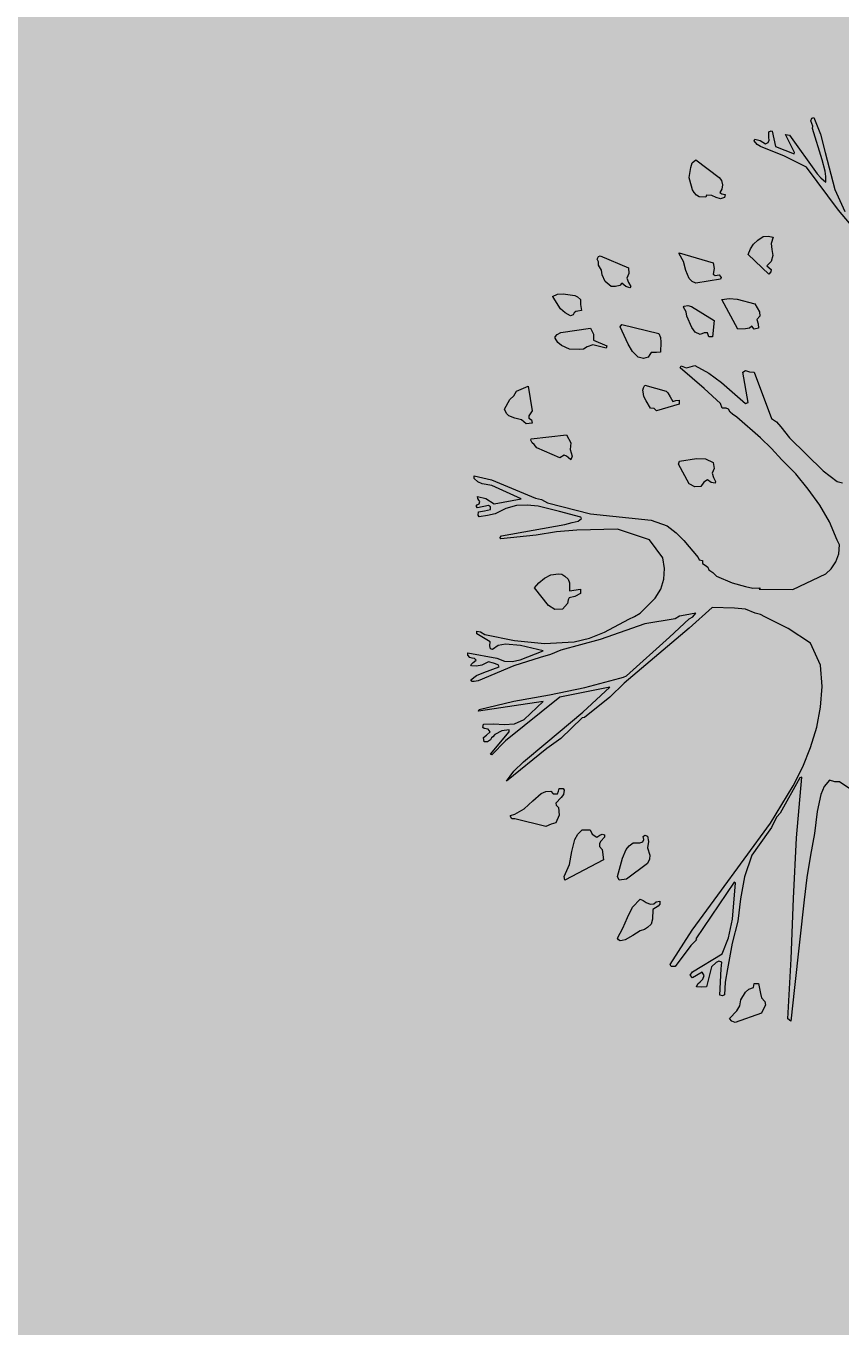
# Model space of a CAD drawing. Units: inches. Extents: x 84 to 1044, y -280 to 906.
# Tile 101 of 105: x 861 to 882, y 478 to 510. Entities that reach past the tile are written whole.
import ezdxf

# ---------------------------------------------------------------- set-up
doc = ezdxf.new("R2010")
doc.units = ezdxf.units.IN
doc.layers.add('A-ANNO-DIMS', color=2, linetype='Continuous', lineweight=18)
doc.layers.add('L-PLNT', color=114, linetype='Continuous', lineweight=15)
doc.layers.add('L-PLNT-PATT', color=9, linetype='Continuous', lineweight=9, true_color=0xafd9aa)
doc.styles.get("Standard").update_dxf_attribs({"font": 'arial.ttf'})
doc.dimstyles.get("Standard").update_dxf_attribs({"dimtxt": 0.18, "dimasz": 0.18, "dimexe": 0.18, "dimexo": 0.0625, "dimgap": 0.09, "dimtad": 0, "dimtih": 1, "dimtoh": 1, "dimdec": 4, "dimzin": 0, "dimdsep": 46, "dimtxsty": 'Standard', "dimcen": 0.09, "dimadec": 0, "dimazin": 0, "dimtfac": 1, "dimtdec": 4, "dimtofl": 0, "dimtmove": 0, "dimatfit": 3, "dimfxl": 1, "dimtolj": 1, "dimtzin": 0, "dimarcsym": 0})

# ---------------------------------------------------------------- blocks, each defined once
blk = doc.blocks.new('A$C37E508DF')
for p, q in [((0.5583, 1.4948), (0.5596, 1.4995)), ((0.5596, 1.4905), (0.5583, 1.4948)), ((0.5596, 1.4995), (0.563, 1.5003)), ((0.5613, 1.4862), (0.5596, 1.4905)), ((0.5608, 1.4823), (0.5613, 1.4862)), ((0.5767, 1.4317), (0.5608, 1.4823)), ((0.563, 1.5003), (0.5737, 1.4733)), ((0.4657, 1.4622), (0.4669, 1.4652)), ((0.4708, 1.4566), (0.4657, 1.4622)), ((0.4669, 1.4652), (0.4755, 1.463)), ((0.4755, 1.463), (0.4845, 1.4575)), ((0.4884, 1.4596), (0.4905, 1.4635)), ((0.4897, 1.4772), (0.4935, 1.4789)), ((0.4897, 1.4678), (0.4897, 1.4772)), ((0.4905, 1.4635), (0.4897, 1.4678)), ((0.4935, 1.4789), (0.4952, 1.478)), ((0.4952, 1.478), (0.5004, 1.4532)), ((0.5313, 1.4437), (0.5167, 1.4729)), ((0.5167, 1.4729), (0.5231, 1.4716)), ((0.5231, 1.4716), (0.5686, 1.409)), ((0.5737, 1.4733), (0.5814, 1.4437)), ((0.4764, 1.4532), (0.4708, 1.4566)), ((0.5154, 1.4373), (0.4764, 1.4532)), ((0.4845, 1.4575), (0.4884, 1.4596)), ((0.5004, 1.4532), (0.5308, 1.4412)), ((0.5308, 1.4412), (0.5313, 1.4437)), ((0.5814, 1.4437), (0.5969, 1.3833)), ((0.3598, 1.403), (0.3628, 1.4189)), ((0.3628, 1.4189), (0.3649, 1.4266)), ((0.3649, 1.4266), (0.3709, 1.4317)), ((0.3709, 1.4317), (0.4086, 1.403)), ((0.551, 1.4197), (0.5154, 1.4373)), ((0.6029, 1.3494), (0.551, 1.4197)), ((0.5814, 1.4133), (0.5767, 1.4317)), ((0.3602, 1.4021), (0.3598, 1.403)), ((0.364, 1.3888), (0.3602, 1.4021)), ((0.4086, 1.403), (0.4125, 1.3979)), ((0.4125, 1.3979), (0.4142, 1.391)), ((0.5686, 1.409), (0.5741, 1.4021)), ((0.5741, 1.4021), (0.5823, 1.3953)), ((0.5827, 1.4043), (0.5814, 1.4133)), ((0.5823, 1.3953), (0.5827, 1.4043)), ((0.3657, 1.3828), (0.364, 1.3888)), ((0.3683, 1.3781), (0.3657, 1.3828)), ((0.3718, 1.3738), (0.3683, 1.3781)), ((0.4134, 1.3837), (0.4099, 1.3781)), ((0.4099, 1.3781), (0.4134, 1.376)), ((0.4142, 1.391), (0.4134, 1.3837)), ((0.4134, 1.376), (0.4189, 1.3751)), ((0.5969, 1.3833), (0.6132, 1.3472)), ((0.3765, 1.3713), (0.3718, 1.3738)), ((0.3872, 1.3708), (0.3765, 1.3713)), ((0.3885, 1.3738), (0.3872, 1.3708)), ((0.3971, 1.3734), (0.3885, 1.3738)), ((0.4039, 1.3704), (0.3971, 1.3734)), ((0.4108, 1.3683), (0.4039, 1.3704)), ((0.4176, 1.37), (0.4108, 1.3683)), ((0.4189, 1.3751), (0.4176, 1.37)), ((0.6595, 1.2829), (0.6029, 1.3494)), ((0.4597, 1.2868), (0.4648, 1.2945)), ((0.4648, 1.2945), (0.4717, 1.3009)), ((0.4717, 1.3009), (0.4807, 1.3065)), ((0.4807, 1.3065), (0.4884, 1.3074)), ((0.4884, 1.3074), (0.4965, 1.3057)), ((0.4965, 1.3057), (0.4935, 1.2954)), ((0.4935, 1.2954), (0.4948, 1.2855)), ((0.2101, 1.2696), (0.2127, 1.2744)), ((0.2127, 1.2744), (0.2152, 1.2752)), ((0.2152, 1.2752), (0.2611, 1.2559)), ((0.3439, 1.2804), (0.3992, 1.2636)), ((0.3439, 1.2787), (0.3439, 1.2804)), ((0.3507, 1.2662), (0.3439, 1.2787)), ((0.4562, 1.2774), (0.4597, 1.2868)), ((0.4897, 1.2452), (0.4562, 1.2774)), ((0.4961, 1.2756), (0.4935, 1.2658)), ((0.4948, 1.2855), (0.4961, 1.2756)), ((0.2127, 1.2654), (0.2101, 1.2696)), ((0.2127, 1.2602), (0.2127, 1.2654)), ((0.2174, 1.2521), (0.2127, 1.2602)), ((0.2182, 1.2443), (0.2174, 1.2521)), ((0.2611, 1.2559), (0.262, 1.2465)), ((0.3546, 1.2516), (0.3507, 1.2662)), ((0.3602, 1.2383), (0.3546, 1.2516)), ((0.3992, 1.2636), (0.4005, 1.2546)), ((0.4005, 1.2546), (0.3992, 1.2452)), ((0.4935, 1.2658), (0.4867, 1.2589)), ((0.4867, 1.2589), (0.4935, 1.2529)), ((0.4931, 1.2491), (0.4897, 1.2452)), ((0.4935, 1.2529), (0.4931, 1.2491)), ((0.2234, 1.2336), (0.2182, 1.2443)), ((0.2328, 1.2251), (0.2234, 1.2336)), ((0.2504, 1.2306), (0.2474, 1.2268)), ((0.2568, 1.2255), (0.2504, 1.2306)), ((0.262, 1.2465), (0.2586, 1.2388)), ((0.2586, 1.2388), (0.2611, 1.2319)), ((0.2611, 1.2319), (0.265, 1.2251)), ((0.3649, 1.2336), (0.3602, 1.2383)), ((0.3709, 1.2306), (0.3649, 1.2336)), ((0.4112, 1.2375), (0.3709, 1.2306)), ((0.3992, 1.2452), (0.4026, 1.2431)), ((0.4026, 1.2431), (0.4086, 1.2443)), ((0.4086, 1.2443), (0.4121, 1.2401)), ((0.4121, 1.2401), (0.4112, 1.2375)), ((0.1376, 1.2092), (0.1458, 1.2126)), ((0.1389, 1.2079), (0.1376, 1.2092)), ((0.1505, 1.189), (0.1389, 1.2079)), ((0.1458, 1.2126), (0.1548, 1.2135)), ((0.1548, 1.2135), (0.1741, 1.2109)), ((0.1741, 1.2109), (0.1784, 1.2083)), ((0.1784, 1.2083), (0.1831, 1.204)), ((0.2401, 1.2251), (0.2328, 1.2251)), ((0.2474, 1.2268), (0.2401, 1.2251)), ((0.2633, 1.2229), (0.2568, 1.2255)), ((0.265, 1.2251), (0.2633, 1.2229)), ((0.1582, 1.1822), (0.1505, 1.189)), ((0.1788, 1.1852), (0.1758, 1.1847)), ((0.1848, 1.1865), (0.1788, 1.1852)), ((0.1831, 1.204), (0.1831, 1.1959)), ((0.1831, 1.1959), (0.1848, 1.1865)), ((0.3507, 1.1916), (0.352, 1.1933)), ((0.355, 1.1839), (0.3507, 1.1916)), ((0.352, 1.1933), (0.3576, 1.1942)), ((0.3576, 1.1942), (0.364, 1.1929)), ((0.364, 1.1929), (0.4005, 1.1702)), ((0.4134, 1.204), (0.4258, 1.2058)), ((0.4391, 1.156), (0.4134, 1.204)), ((0.4258, 1.2058), (0.4382, 1.2045)), ((0.4382, 1.2045), (0.4669, 1.1972)), ((0.4669, 1.1972), (0.4747, 1.1843)), ((0.1668, 1.1775), (0.1582, 1.1822)), ((0.1711, 1.1792), (0.1668, 1.1775)), ((0.1728, 1.1826), (0.1711, 1.1792)), ((0.1758, 1.1847), (0.1728, 1.1826)), ((0.3563, 1.177), (0.355, 1.1839)), ((0.3645, 1.1586), (0.3563, 1.177)), ((0.4005, 1.1702), (0.3979, 1.1436)), ((0.4751, 1.177), (0.47, 1.1714)), ((0.47, 1.1714), (0.4721, 1.1646)), ((0.4721, 1.1646), (0.473, 1.1573)), ((0.4747, 1.1843), (0.4751, 1.177)), ((0.1419, 1.1436), (0.1449, 1.1474)), ((0.1419, 1.141), (0.1419, 1.1436)), ((0.1449, 1.1474), (0.1509, 1.1504)), ((0.1509, 1.1504), (0.1994, 1.1573)), ((0.1994, 1.1573), (0.2041, 1.1479)), ((0.2041, 1.1479), (0.2045, 1.138)), ((0.2478, 1.1594), (0.2504, 1.1637)), ((0.2607, 1.1316), (0.2478, 1.1594)), ((0.2504, 1.1637), (0.3104, 1.1487)), ((0.3104, 1.1487), (0.3134, 1.1423)), ((0.37, 1.1509), (0.3645, 1.1586)), ((0.3778, 1.1474), (0.37, 1.1509)), ((0.3842, 1.15), (0.3778, 1.1474)), ((0.3898, 1.15), (0.3842, 1.15)), ((0.3923, 1.1436), (0.3898, 1.15)), ((0.3979, 1.1436), (0.3923, 1.1436)), ((0.4519, 1.1564), (0.4391, 1.156)), ((0.458, 1.1573), (0.4519, 1.1564)), ((0.4622, 1.1607), (0.458, 1.1573)), ((0.4657, 1.156), (0.4622, 1.1607)), ((0.473, 1.1573), (0.4657, 1.156)), ((0.1462, 1.1342), (0.1419, 1.141)), ((0.1522, 1.1294), (0.1462, 1.1342)), ((0.1655, 1.1234), (0.1522, 1.1294)), ((0.181, 1.1226), (0.1655, 1.1234)), ((0.1878, 1.1234), (0.181, 1.1226)), ((0.1938, 1.1273), (0.1878, 1.1234)), ((0.2032, 1.1303), (0.1938, 1.1273)), ((0.2247, 1.1251), (0.2032, 1.1303)), ((0.2045, 1.138), (0.226, 1.129)), ((0.226, 1.129), (0.2247, 1.1251)), ((0.268, 1.1196), (0.2607, 1.1316)), ((0.3134, 1.1423), (0.3139, 1.1346)), ((0.3139, 1.1346), (0.3134, 1.1183)), ((0.277, 1.1101), (0.268, 1.1196)), ((0.2856, 1.108), (0.277, 1.1101)), ((0.2933, 1.1101), (0.2856, 1.108)), ((0.2959, 1.1144), (0.2933, 1.1101)), ((0.2984, 1.1179), (0.2959, 1.1144)), ((0.3066, 1.1179), (0.2984, 1.1179)), ((0.3134, 1.1183), (0.3066, 1.1179)), ((0.3456, 1.093), (0.3469, 1.0964)), ((0.3842, 1.0591), (0.3456, 1.093)), ((0.3469, 1.0964), (0.355, 1.093)), ((0.355, 1.093), (0.3619, 1.0943)), ((0.3619, 1.0943), (0.3692, 1.0968)), ((0.3692, 1.0968), (0.3923, 1.0844)), ((0.3923, 1.0844), (0.4129, 1.069)), ((0.4472, 1.0857), (0.4515, 1.0887)), ((0.4562, 1.0364), (0.4472, 1.0857)), ((0.4515, 1.0887), (0.4584, 1.0865)), ((0.4584, 1.0865), (0.4657, 1.0861)), ((0.4657, 1.0861), (0.4939, 1.0107)), ((0.0789, 1.0552), (0.0978, 1.063)), ((0.0978, 1.063), (0.1042, 1.0231)), ((0.2847, 1.0565), (0.2856, 1.0604)), ((0.2856, 1.0604), (0.2877, 1.0647)), ((0.2877, 1.0647), (0.3224, 1.0552)), ((0.4112, 1.0351), (0.3842, 1.0591)), ((0.4129, 1.069), (0.4515, 1.0351)), ((0.0596, 1.0257), (0.0682, 1.0415)), ((0.0682, 1.0415), (0.0746, 1.0475)), ((0.0746, 1.0475), (0.0789, 1.0552)), ((0.2851, 1.054), (0.2847, 1.0565)), ((0.2864, 1.0463), (0.2851, 1.054)), ((0.2899, 1.039), (0.2864, 1.0463)), ((0.2972, 1.0274), (0.2899, 1.039)), ((0.3224, 1.0552), (0.3255, 1.0522)), ((0.3255, 1.0522), (0.3293, 1.0458)), ((0.3293, 1.0458), (0.3336, 1.0381)), ((0.3336, 1.0381), (0.3383, 1.0398)), ((0.3383, 1.0398), (0.3439, 1.0402)), ((0.3439, 1.0402), (0.3439, 1.0338)), ((0.0626, 1.0188), (0.0596, 1.0257)), ((0.0665, 1.0149), (0.0626, 1.0188)), ((0.1012, 1.018), (0.099, 1.0149)), ((0.1042, 1.0231), (0.1012, 1.018)), ((0.3032, 1.0265), (0.2972, 1.0274)), ((0.3066, 1.0231), (0.3032, 1.0265)), ((0.3439, 1.0338), (0.3066, 1.0231)), ((0.4138, 1.0274), (0.4112, 1.0351)), ((0.4202, 1.0274), (0.4138, 1.0274)), ((0.4241, 1.0257), (0.4202, 1.0274)), ((0.4267, 1.0209), (0.4241, 1.0257)), ((0.4305, 1.0175), (0.4267, 1.0209)), ((0.4378, 1.0124), (0.4305, 1.0175)), ((0.4515, 1.0351), (0.4562, 1.0364)), ((0.0763, 1.0111), (0.0665, 1.0149)), ((0.087, 1.0085), (0.0763, 1.0111)), ((0.0948, 1.0016), (0.087, 1.0085)), ((0.1042, 1.0029), (0.0948, 1.0016)), ((0.099, 1.0149), (0.099, 1.0111)), ((0.099, 1.0111), (0.1033, 1.0085)), ((0.1033, 1.0085), (0.1042, 1.0029)), ((0.476, 0.9789), (0.4378, 1.0124)), ((0.4939, 1.0107), (0.5021, 1.0051)), ((0.5021, 1.0051), (0.5094, 0.9969)), ((0.5094, 0.9969), (0.5231, 0.9789)), ((0.1025, 0.9751), (0.1029, 0.9772)), ((0.1046, 0.9708), (0.1025, 0.9751)), ((0.1029, 0.9772), (0.1604, 0.9841)), ((0.1604, 0.9841), (0.1672, 0.9708)), ((0.4939, 0.9618), (0.476, 0.9789)), ((0.5231, 0.9789), (0.578, 0.9253)), ((0.1076, 0.9682), (0.1046, 0.9708)), ((0.1119, 0.9626), (0.1076, 0.9682)), ((0.1496, 0.9463), (0.1119, 0.9626)), ((0.1672, 0.9708), (0.1664, 0.9601)), ((0.1664, 0.9601), (0.1698, 0.9493)), ((0.5111, 0.9429), (0.4939, 0.9618)), ((0.1565, 0.9506), (0.1496, 0.9463)), ((0.1604, 0.9493), (0.1565, 0.9506)), ((0.1629, 0.9468), (0.1604, 0.9493)), ((0.1672, 0.9429), (0.1629, 0.9468)), ((0.1698, 0.9493), (0.1672, 0.9429)), ((0.3426, 0.936), (0.3443, 0.9412)), ((0.3602, 0.9039), (0.3426, 0.936)), ((0.3443, 0.9412), (0.3722, 0.9451)), ((0.3722, 0.9451), (0.3868, 0.9446)), ((0.3868, 0.9446), (0.3992, 0.9386)), ((0.3992, 0.9386), (0.4009, 0.9292)), ((0.5334, 0.9202), (0.5111, 0.9429)), ((0.0103, 0.9129), (0.0103, 0.9172)), ((0.0103, 0.9172), (0.0382, 0.9107)), ((0.0159, 0.9073), (0.0103, 0.9129)), ((0.0382, 0.9107), (0.1098, 0.8807)), ((0.3898, 0.9107), (0.3838, 0.9069)), ((0.3958, 0.906), (0.3898, 0.9107)), ((0.4009, 0.9292), (0.3975, 0.9215)), ((0.3975, 0.9215), (0.3996, 0.9142)), ((0.3996, 0.9142), (0.4031, 0.9077)), ((0.554, 0.8953), (0.5334, 0.9202)), ((0.578, 0.9253), (0.6011, 0.9077)), ((0.0232, 0.9043), (0.0159, 0.9073)), ((0.0386, 0.9013), (0.0232, 0.9043)), ((0.0866, 0.8794), (0.0386, 0.9013)), ((0.3692, 0.8992), (0.3602, 0.9039)), ((0.379, 0.9), (0.3692, 0.8992)), ((0.3838, 0.9069), (0.379, 0.9)), ((0.4026, 0.9052), (0.3958, 0.906)), ((0.4031, 0.9077), (0.4026, 0.9052)), ((0.5728, 0.8691), (0.554, 0.8953)), ((0.6011, 0.9077), (0.6097, 0.9056)), ((0.0133, 0.8679), (0.015, 0.87)), ((0.0154, 0.8649), (0.0133, 0.8679)), ((0.015, 0.87), (0.0184, 0.8717)), ((0.0159, 0.8803), (0.0154, 0.8837)), ((0.0154, 0.8837), (0.0292, 0.8803)), ((0.0334, 0.8687), (0.0154, 0.8649)), ((0.0176, 0.8777), (0.0159, 0.8803)), ((0.0193, 0.8752), (0.0176, 0.8777)), ((0.0184, 0.8717), (0.0193, 0.8752)), ((0.0292, 0.8803), (0.0424, 0.8717)), ((0.0369, 0.8666), (0.0334, 0.8687)), ((0.0424, 0.8717), (0.0866, 0.8794)), ((0.0789, 0.8687), (0.0617, 0.864)), ((0.0965, 0.8696), (0.0789, 0.8687)), ((0.1141, 0.8679), (0.0965, 0.8696)), ((0.1098, 0.8807), (0.1196, 0.8786)), ((0.1492, 0.8593), (0.1141, 0.8679)), ((0.1196, 0.8786), (0.1295, 0.873)), ((0.1295, 0.873), (0.1994, 0.8554)), ((0.5887, 0.8421), (0.5728, 0.8691)), ((0.0163, 0.8529), (0.0171, 0.8584)), ((0.0184, 0.8503), (0.0163, 0.8529)), ((0.0171, 0.8584), (0.0266, 0.8602)), ((0.0317, 0.8524), (0.0184, 0.8503)), ((0.0266, 0.8602), (0.0369, 0.8623)), ((0.0442, 0.8554), (0.0317, 0.8524)), ((0.0369, 0.8623), (0.0369, 0.8666)), ((0.0617, 0.864), (0.0442, 0.8554)), ((0.1835, 0.8499), (0.1492, 0.8593)), ((0.1792, 0.8434), (0.1848, 0.8477)), ((0.1848, 0.8477), (0.1835, 0.8499)), ((0.1994, 0.8554), (0.2984, 0.8447)), ((0.0545, 0.8194), (0.1578, 0.8378)), ((0.1441, 0.8258), (0.1111, 0.8207)), ((0.1771, 0.8288), (0.1441, 0.8258)), ((0.1578, 0.8378), (0.1698, 0.8413)), ((0.1698, 0.8413), (0.1792, 0.8434)), ((0.2436, 0.8301), (0.1771, 0.8288)), ((0.2954, 0.813), (0.2436, 0.8301)), ((0.2984, 0.8447), (0.3242, 0.8357)), ((0.3242, 0.8357), (0.3387, 0.8241)), ((0.6007, 0.8125), (0.5887, 0.8421)), ((0.0519, 0.8164), (0.0545, 0.8194)), ((0.0532, 0.8143), (0.0519, 0.8164)), ((0.1111, 0.8207), (0.0532, 0.8143)), ((0.3173, 0.7834), (0.2954, 0.813)), ((0.3387, 0.8241), (0.3512, 0.8117)), ((0.3512, 0.8117), (0.3748, 0.7842)), ((0.6046, 0.8048), (0.6007, 0.8125)), ((0.6037, 0.7903), (0.6046, 0.8048)), ((0.3199, 0.7662), (0.3173, 0.7834)), ((0.3748, 0.7842), (0.3765, 0.7804)), ((0.599, 0.777), (0.6037, 0.7903)), ((0.3186, 0.7491), (0.3199, 0.7662)), ((0.3765, 0.7804), (0.3816, 0.7791)), ((0.3816, 0.7791), (0.382, 0.7744)), ((0.382, 0.7744), (0.3859, 0.7714)), ((0.3859, 0.7714), (0.3902, 0.7684)), ((0.3902, 0.7684), (0.3919, 0.7641)), ((0.3919, 0.7641), (0.3988, 0.7598)), ((0.5823, 0.7577), (0.5913, 0.7658)), ((0.5913, 0.7658), (0.599, 0.777)), ((0.1081, 0.7349), (0.1153, 0.7427)), ((0.1153, 0.7427), (0.1244, 0.7504)), ((0.1244, 0.7504), (0.1351, 0.7559)), ((0.1351, 0.7559), (0.1471, 0.7577)), ((0.1471, 0.7577), (0.1527, 0.7568)), ((0.1527, 0.7568), (0.1578, 0.7538)), ((0.1578, 0.7538), (0.1629, 0.7491)), ((0.1629, 0.7491), (0.1651, 0.7431)), ((0.1651, 0.7431), (0.1655, 0.7298)), ((0.3139, 0.7324), (0.3186, 0.7491)), ((0.3988, 0.7598), (0.4043, 0.7538)), ((0.4043, 0.7538), (0.4301, 0.7431)), ((0.4301, 0.7431), (0.4515, 0.7371)), ((0.5287, 0.7319), (0.5823, 0.7577)), ((0.1312, 0.7058), (0.1081, 0.7349)), ((0.1741, 0.7208), (0.1646, 0.7186)), ((0.1655, 0.7298), (0.1831, 0.7324)), ((0.1831, 0.7255), (0.1741, 0.7208)), ((0.1831, 0.7324), (0.1831, 0.7255)), ((0.3049, 0.7178), (0.3139, 0.7324)), ((0.4515, 0.7371), (0.4635, 0.7341)), ((0.4635, 0.7341), (0.4755, 0.7349)), ((0.4755, 0.7349), (0.4742, 0.7324)), ((0.4742, 0.7324), (0.5287, 0.7319)), ((0.1415, 0.6994), (0.1312, 0.7058)), ((0.1539, 0.7002), (0.1415, 0.6994)), ((0.1621, 0.7092), (0.1539, 0.7002)), ((0.1629, 0.7152), (0.1621, 0.7092)), ((0.1646, 0.7186), (0.1629, 0.7152)), ((0.28, 0.6933), (0.3049, 0.7178)), ((0.3975, 0.7028), (0.3598, 0.6693)), ((0.4339, 0.7019), (0.3975, 0.7028)), ((0.4515, 0.7002), (0.4339, 0.7019)), ((0.4674, 0.6933), (0.4515, 0.7002)), ((0.2221, 0.6625), (0.262, 0.6839)), ((0.262, 0.6839), (0.271, 0.6882)), ((0.271, 0.6882), (0.28, 0.6933)), ((0.337, 0.6843), (0.2877, 0.6762)), ((0.328, 0.6543), (0.3598, 0.6843)), ((0.3443, 0.6886), (0.337, 0.6843)), ((0.3533, 0.6903), (0.3443, 0.6886)), ((0.3709, 0.6933), (0.3533, 0.6903)), ((0.3598, 0.6843), (0.3662, 0.6873)), ((0.3662, 0.6873), (0.3709, 0.6933)), ((0.476, 0.6912), (0.4674, 0.6933)), ((0.4832, 0.6878), (0.476, 0.6912)), ((0.521, 0.6685), (0.4832, 0.6878)), ((0.0146, 0.6599), (0.0146, 0.6642)), ((0.0146, 0.6642), (0.0206, 0.6633)), ((0.036, 0.6466), (0.0146, 0.6599)), ((0.0206, 0.6633), (0.0274, 0.6586)), ((0.0274, 0.6586), (0.0759, 0.6492)), ((0.1977, 0.6526), (0.2221, 0.6625)), ((0.2877, 0.6762), (0.2152, 0.6505)), ((0.3598, 0.6693), (0.2543, 0.5797)), ((0.5578, 0.6449), (0.521, 0.6685)), ((0.0356, 0.6406), (0.036, 0.6466)), ((0.0369, 0.6355), (0.0356, 0.6406)), ((0.0399, 0.6342), (0.0369, 0.6355)), ((0.0489, 0.641), (0.0399, 0.6342)), ((0.0609, 0.6428), (0.0489, 0.641)), ((0.0853, 0.641), (0.0609, 0.6428)), ((0.0759, 0.6492), (0.1244, 0.644)), ((0.1226, 0.632), (0.0853, 0.641)), ((0.1244, 0.644), (0.1728, 0.647)), ((0.2152, 0.6505), (0.1509, 0.6333)), ((0.1728, 0.647), (0.1977, 0.6526)), ((0.2581, 0.5913), (0.328, 0.6543)), ((0.5737, 0.6089), (0.5578, 0.6449)), ((0, 0.629), (0.0467, 0.62)), ((0, 0.6252), (0, 0.629)), ((0.003, 0.6213), (0, 0.6252)), ((0.0069, 0.6204), (0.003, 0.6213)), ((0.0107, 0.6196), (0.0069, 0.6204)), ((0.0086, 0.6132), (0.0133, 0.617)), ((0.0133, 0.617), (0.0107, 0.6196)), ((0.0334, 0.6145), (0.0223, 0.6089)), ((0.0416, 0.6119), (0.0334, 0.6145)), ((0.0467, 0.62), (0.0592, 0.6153)), ((0.0592, 0.6153), (0.072, 0.6149)), ((0.072, 0.6149), (0.0849, 0.6175)), ((0.1175, 0.6213), (0.0746, 0.6076)), ((0.0849, 0.6175), (0.0973, 0.6226)), ((0.0973, 0.6226), (0.1226, 0.632)), ((0.1342, 0.6265), (0.1175, 0.6213)), ((0.1509, 0.6333), (0.1342, 0.6265)), ((0.0047, 0.6093), (0.0086, 0.6132)), ((0.0056, 0.6076), (0.0047, 0.6093)), ((0.0141, 0.6072), (0.0056, 0.6076)), ((0.0223, 0.6089), (0.0141, 0.6072)), ((0.0141, 0.5921), (0.0257, 0.5969)), ((0.0746, 0.6076), (0.0163, 0.5836)), ((0.0257, 0.5969), (0.0506, 0.6063)), ((0.0493, 0.6093), (0.0416, 0.6119)), ((0.0506, 0.6063), (0.0493, 0.6093)), ((0.5763, 0.5741), (0.5737, 0.6089)), ((0.0047, 0.5849), (0.0141, 0.5921)), ((0.0069, 0.5823), (0.0047, 0.5849)), ((0.0099, 0.5823), (0.0069, 0.5823)), ((0.0163, 0.5836), (0.0099, 0.5823)), ((0.1325, 0.5608), (0.1904, 0.5724)), ((0.2311, 0.5729), (0.1496, 0.557)), ((0.1869, 0.5325), (0.2311, 0.5729)), ((0.1904, 0.5724), (0.2474, 0.5879)), ((0.2543, 0.5797), (0.2311, 0.557)), ((0.2474, 0.5879), (0.253, 0.5892)), ((0.253, 0.5892), (0.2581, 0.5913)), ((0.5737, 0.5407), (0.5763, 0.5741)), ((0.1496, 0.557), (0.0613, 0.4858)), ((0.0746, 0.5501), (0.1325, 0.5608)), ((0.2311, 0.557), (0.1899, 0.5235)), ((0.1226, 0.5497), (0.0171, 0.5338)), ((0.0171, 0.5338), (0.0184, 0.5368)), ((0.0184, 0.5368), (0.0746, 0.5501)), ((0.0917, 0.5205), (0.1226, 0.5497)), ((0.1269, 0.482), (0.1869, 0.5325)), ((0.5677, 0.5077), (0.5737, 0.5407)), ((0.024, 0.5072), (0.0253, 0.5128)), ((0.0253, 0.5128), (0.042, 0.5133)), ((0.042, 0.5133), (0.0587, 0.5124)), ((0.0587, 0.5124), (0.0755, 0.5133)), ((0.0755, 0.5133), (0.0917, 0.5205)), ((0.1861, 0.5231), (0.1509, 0.4897)), ((0.1899, 0.5235), (0.1861, 0.5231)), ((0.0262, 0.5055), (0.024, 0.5072)), ((0.0253, 0.491), (0.03, 0.4948)), ((0.0262, 0.4841), (0.0253, 0.491)), ((0.0326, 0.5047), (0.0262, 0.5055)), ((0.03, 0.4948), (0.036, 0.5004)), ((0.0369, 0.4871), (0.0317, 0.4841)), ((0.036, 0.5004), (0.0326, 0.5047)), ((0.0369, 0.4639), (0.0669, 0.5004)), ((0.0382, 0.4905), (0.0369, 0.4871)), ((0.0403, 0.4922), (0.0382, 0.4905)), ((0.0437, 0.4961), (0.0403, 0.4922)), ((0.0549, 0.5021), (0.0437, 0.4961)), ((0.0669, 0.5034), (0.0549, 0.5021)), ((0.0669, 0.5004), (0.0669, 0.5034)), ((0.1509, 0.4897), (0.1282, 0.4734)), ((0.5578, 0.4751), (0.5677, 0.5077)), ((0.0317, 0.4841), (0.0262, 0.4841)), ((0.0613, 0.4858), (0.0386, 0.4627)), ((0.1282, 0.4734), (0.0626, 0.4198)), ((0.0905, 0.4515), (0.1269, 0.482)), ((0.545, 0.4434), (0.5578, 0.4751)), ((0.0386, 0.4627), (0.0369, 0.4639)), ((0.0746, 0.4361), (0.0905, 0.4515)), ((0.0626, 0.4198), (0.0746, 0.4361)), ((0.5403, 0.4254), (0.5081, 0.3679)), ((0.5295, 0.4125), (0.545, 0.4434)), ((0.5347, 0.3276), (0.5433, 0.4266)), ((0.5433, 0.4266), (0.5403, 0.4254)), ((0.1192, 0.4001), (0.1265, 0.4031)), ((0.1265, 0.4031), (0.1346, 0.4039)), ((0.1346, 0.4039), (0.1389, 0.3992)), ((0.1458, 0.3996), (0.1471, 0.4035)), ((0.1471, 0.4035), (0.1484, 0.4082)), ((0.1484, 0.4082), (0.1548, 0.4082)), ((0.1548, 0.4082), (0.1565, 0.4052)), ((0.1565, 0.4052), (0.1556, 0.3983)), ((0.4922, 0.3516), (0.5295, 0.4125)), ((0.5797, 0.4112), (0.5741, 0.3983)), ((0.5887, 0.4215), (0.5797, 0.4112)), ((0.5969, 0.4189), (0.5887, 0.4215)), ((0.6046, 0.4189), (0.5969, 0.4189)), ((0.6295, 0.4022), (0.6046, 0.4189)), ((0.0917, 0.3748), (0.1055, 0.388)), ((0.1055, 0.388), (0.1192, 0.4001)), ((0.1389, 0.3992), (0.1458, 0.3996)), ((0.1518, 0.3932), (0.1432, 0.3842)), ((0.1432, 0.3842), (0.1436, 0.3808)), ((0.1556, 0.3983), (0.1518, 0.3932)), ((0.5741, 0.3983), (0.5686, 0.3705)), ((0.069, 0.364), (0.0763, 0.3662)), ((0.069, 0.3627), (0.069, 0.364)), ((0.0716, 0.3585), (0.069, 0.3627)), ((0.0763, 0.3662), (0.0917, 0.3748)), ((0.1484, 0.3649), (0.1432, 0.352)), ((0.1436, 0.3808), (0.1471, 0.3769)), ((0.1471, 0.3769), (0.1484, 0.3649)), ((0.5025, 0.3619), (0.4982, 0.3537)), ((0.5081, 0.3679), (0.5025, 0.3619)), ((0.5686, 0.3705), (0.5643, 0.3349)), ((0.0763, 0.3585), (0.0716, 0.3585)), ((0.1269, 0.3464), (0.0763, 0.3585)), ((0.1355, 0.3499), (0.1269, 0.3464)), ((0.1432, 0.352), (0.1355, 0.3499)), ((0.1788, 0.3336), (0.1861, 0.3409)), ((0.1861, 0.3409), (0.199, 0.3409)), ((0.199, 0.3409), (0.2024, 0.3336)), ((0.4065, 0.2345), (0.4922, 0.3516)), ((0.4939, 0.3447), (0.4884, 0.337)), ((0.4982, 0.3537), (0.4939, 0.3447)), ((0.1689, 0.3053), (0.1737, 0.325)), ((0.1737, 0.325), (0.1788, 0.3336)), ((0.2024, 0.3336), (0.2097, 0.3289)), ((0.2097, 0.3289), (0.2148, 0.3323)), ((0.2161, 0.3224), (0.214, 0.3186)), ((0.214, 0.3186), (0.214, 0.3139)), ((0.2148, 0.3323), (0.2182, 0.3336)), ((0.2221, 0.3289), (0.2161, 0.3224)), ((0.2182, 0.3336), (0.2221, 0.3327)), ((0.2221, 0.3327), (0.2221, 0.3289)), ((0.2624, 0.3147), (0.2689, 0.3194)), ((0.2689, 0.3194), (0.2796, 0.3194)), ((0.2796, 0.3194), (0.2847, 0.3211)), ((0.2847, 0.3211), (0.2864, 0.325)), ((0.2851, 0.3302), (0.2877, 0.3319)), ((0.2864, 0.325), (0.2851, 0.3302)), ((0.2877, 0.3319), (0.292, 0.3306)), ((0.292, 0.3306), (0.2941, 0.322)), ((0.2941, 0.322), (0.292, 0.3117)), ((0.4884, 0.337), (0.4622, 0.2997)), ((0.53, 0.229), (0.5347, 0.3276)), ((0.5643, 0.3349), (0.5578, 0.2993)), ((0.1655, 0.2843), (0.1689, 0.3053)), ((0.214, 0.3139), (0.2182, 0.3087)), ((0.2182, 0.3087), (0.2204, 0.292)), ((0.2517, 0.2946), (0.2577, 0.3087)), ((0.2577, 0.3087), (0.2624, 0.3147)), ((0.292, 0.3117), (0.2959, 0.2993)), ((0.2959, 0.2993), (0.2954, 0.2928)), ((0.4622, 0.2997), (0.4502, 0.2645)), ((0.5578, 0.2993), (0.5518, 0.2633)), ((0.1565, 0.265), (0.1655, 0.2843)), ((0.2204, 0.292), (0.1578, 0.259)), ((0.2436, 0.265), (0.2517, 0.2946)), ((0.292, 0.286), (0.2581, 0.2607)), ((0.2954, 0.2928), (0.292, 0.286)), ((0.1578, 0.259), (0.1565, 0.265)), ((0.2461, 0.259), (0.2436, 0.265)), ((0.2581, 0.2607), (0.2461, 0.259)), ((0.4335, 0.2556), (0.3709, 0.1634)), ((0.4305, 0.1951), (0.4352, 0.2543)), ((0.4352, 0.2543), (0.4335, 0.2556)), ((0.4502, 0.2645), (0.4438, 0.2285)), ((0.5518, 0.2633), (0.5475, 0.2268)), ((0.3649, 0.1775), (0.4065, 0.2345)), ((0.2594, 0.1981), (0.268, 0.2148)), ((0.268, 0.2148), (0.28, 0.2277)), ((0.28, 0.2277), (0.2851, 0.226)), ((0.2851, 0.226), (0.2903, 0.2225)), ((0.2903, 0.2225), (0.2963, 0.22)), ((0.2963, 0.22), (0.3027, 0.2204)), ((0.3096, 0.2165), (0.301, 0.211)), ((0.3027, 0.2204), (0.3061, 0.2234)), ((0.3061, 0.2234), (0.3122, 0.2247)), ((0.3122, 0.22), (0.3096, 0.2165)), ((0.3122, 0.2247), (0.3122, 0.22)), ((0.4438, 0.2285), (0.4391, 0.1921)), ((0.5261, 0.1308), (0.53, 0.229)), ((0.5475, 0.2268), (0.5313, 0.084)), ((0.2521, 0.1805), (0.2594, 0.1981)), ((0.3002, 0.1951), (0.298, 0.1874)), ((0.301, 0.211), (0.3002, 0.1951)), ((0.4241, 0.1651), (0.4305, 0.1951)), ((0.4391, 0.1921), (0.4301, 0.1561)), ((0.2436, 0.1642), (0.2521, 0.1805)), ((0.28, 0.1762), (0.2684, 0.1689)), ((0.2873, 0.1788), (0.28, 0.1762)), ((0.292, 0.1818), (0.2873, 0.1788)), ((0.298, 0.1874), (0.292, 0.1818)), ((0.3293, 0.1213), (0.3649, 0.1775)), ((0.2448, 0.1616), (0.2436, 0.1642)), ((0.2478, 0.1599), (0.2448, 0.1616)), ((0.2508, 0.1608), (0.2478, 0.1599)), ((0.2556, 0.1616), (0.2508, 0.1608)), ((0.2684, 0.1689), (0.2556, 0.1616)), ((0.3628, 0.1526), (0.337, 0.1183)), ((0.3692, 0.1591), (0.3628, 0.1526)), ((0.3718, 0.1616), (0.3692, 0.1591)), ((0.3709, 0.1634), (0.3718, 0.1616)), ((0.4138, 0.1389), (0.4241, 0.1651)), ((0.4301, 0.1561), (0.4224, 0.1145)), ((0.3653, 0.1098), (0.4138, 0.1389)), ((0.5205, 0.033), (0.5261, 0.1308)), ((0.3306, 0.1183), (0.3293, 0.1213)), ((0.337, 0.1183), (0.3306, 0.1183)), ((0.3615, 0.1042), (0.3653, 0.1098)), ((0.3812, 0.1089), (0.3653, 0.0999)), ((0.3842, 0.1037), (0.3812, 0.1089)), ((0.3962, 0.1175), (0.3885, 0.0853)), ((0.4039, 0.1248), (0.3962, 0.1175)), ((0.4082, 0.1269), (0.4039, 0.1248)), ((0.4134, 0.1256), (0.4082, 0.1269)), ((0.4099, 0.0716), (0.4121, 0.1145)), ((0.4121, 0.1145), (0.4134, 0.1256)), ((0.4224, 0.1145), (0.4189, 0.093)), ((0.3653, 0.0999), (0.3615, 0.1042)), ((0.3722, 0.0853), (0.3739, 0.09)), ((0.3808, 0.0845), (0.3722, 0.0853)), ((0.3739, 0.09), (0.3782, 0.0935)), ((0.3782, 0.0935), (0.3825, 0.0978)), ((0.3885, 0.0853), (0.3808, 0.0845)), ((0.3825, 0.0978), (0.3842, 0.1037)), ((0.4189, 0.093), (0.4176, 0.072)), ((0.4648, 0.084), (0.4657, 0.0905)), ((0.4657, 0.0905), (0.473, 0.0905)), ((0.473, 0.0905), (0.476, 0.0746)), ((0.4142, 0.0707), (0.4099, 0.0716)), ((0.4176, 0.072), (0.4142, 0.0707)), ((0.4425, 0.0544), (0.4442, 0.0639)), ((0.4442, 0.0639), (0.4515, 0.0763)), ((0.4515, 0.0763), (0.4571, 0.0815)), ((0.4571, 0.0815), (0.4648, 0.084)), ((0.476, 0.0746), (0.4777, 0.0673)), ((0.4777, 0.0673), (0.4832, 0.0613)), ((0.5313, 0.084), (0.5257, 0.0291)), ((0.4258, 0.0339), (0.4378, 0.0463)), ((0.4777, 0.0424), (0.4348, 0.0274)), ((0.4378, 0.0463), (0.4425, 0.0544)), ((0.4811, 0.0493), (0.4777, 0.0424)), ((0.4845, 0.0553), (0.4811, 0.0493)), ((0.4832, 0.0613), (0.4845, 0.0553)), ((0.4296, 0.0291), (0.4258, 0.0339)), ((0.4348, 0.0274), (0.4296, 0.0291)), ((0.5257, 0.0291), (0.5205, 0.033))]:
    blk.add_line(p, q)
blk = doc.blocks.new('*D62')
at = {"layer": 'A-ANNO-DIMS', "color": 0, "lineweight": -2, "transparency": 16777216}
for p, q in [((203.179, 709.183), (203.179, 905.9)), ((203.359, 905.72), (549.232, 905.72)), ((895.894, 905.72), (550.021, 905.72)), ((896.074, 400.183), (896.074, 905.9))]:
    blk.add_line(p, q, dxfattribs=at)
at = {"layer": 'A-ANNO-DIMS', "color": 0, "transparency": 16777216}
for points in [[(203.359, 905.75), (203.359, 905.69), (203.179, 905.72)], [(895.894, 905.75), (895.894, 905.69), (896.074, 905.72)]]:
    blk.add_solid(points, dxfattribs=at)
at = {"layer": 'Defpoints', "color": 0, "transparency": 16777216}
for p in [(896.074, 905.72), (203.179, 709.12), (896.074, 400.12)]:
    blk.add_point(p, dxfattribs=at)
at = {"layer": 'A-ANNO-DIMS', "color": 0, "transparency": 16777216, "insert": (549.627, 905.72), "char_height": 0.18, "attachment_point": 5}
blk.add_mtext('\\A1;692.9', dxfattribs=at)
blk = doc.blocks.new('*D63')
at = {"layer": 'A-ANNO-DIMS', "color": 0, "lineweight": -2, "transparency": 16777216}
for p, q in [((833.136, 709.12), (1043.768, 709.12)), ((1043.588, 708.94), (1043.588, 400.302)), ((1043.588, 91.3), (1043.588, 399.938)), ((896.136, 91.12), (1043.768, 91.12))]:
    blk.add_line(p, q, dxfattribs=at)
at = {"layer": 'A-ANNO-DIMS', "color": 0, "transparency": 16777216}
for points in [[(1043.558, 708.94), (1043.618, 708.94), (1043.588, 709.12)], [(1043.558, 91.3), (1043.618, 91.3), (1043.588, 91.12)]]:
    blk.add_solid(points, dxfattribs=at)
at = {"layer": 'Defpoints', "color": 0, "transparency": 16777216}
for p in [(833.074, 709.12), (1043.588, 709.12), (896.074, 91.12)]:
    blk.add_point(p, dxfattribs=at)
at = {"layer": 'A-ANNO-DIMS', "color": 0, "transparency": 16777216, "insert": (1043.588, 400.12), "char_height": 0.18, "attachment_point": 5}
blk.add_mtext('\\A1;618', dxfattribs=at)

msp = doc.modelspace()

# ---------------------------------------------------------------- hatches: boundary and pattern name
at = {"layer": 'L-PLNT-PATT', "transparency": 33554597}
h = msp.add_hatch(color=256, dxfattribs=at)
h.dxf.hatch_style = 1
h.paths.add_polyline_path([(896.074, 511.12), (704.074, 511.12), (704.074, 491.62), (704.074, 419.62), (704.074, 400.12), (833.074, 400.12), (896.074, 400.12)])

# ---------------------------------------------------------------- block references
at = {"layer": 'L-PLNT', "xscale": 15.19586232982809, "yscale": 15.19586232982809, "zscale": 15.19586232982809}
msp.add_blockref('A$C37E508DF', (872.33, 484.736), dxfattribs=at)

# ---------------------------------------------------------------- dimensions: what is measured, and where the dimension line sits
at = {"layer": 'A-ANNO-DIMS'}
dim = msp.add_linear_dim(base=(896.074, 905.72), p1=(203.179, 709.12), p2=(896.074, 400.12), dimstyle='Standard', override={"dimdec": 1, "dimlfac": 1, "dimrnd": 0, "dimzin": 0, "dimdsep": 46, "dimlunit": 2}, dxfattribs=at)
dim.commit()
dim.dimension.update_dxf_attribs({"geometry": '*D62', "text_midpoint": (549.627, 905.72)})
dim = msp.add_linear_dim(base=(1043.588, 709.12), p1=(896.074, 91.12), p2=(833.074, 709.12), angle=90, dimstyle='Standard', override={"dimdec": 0, "dimlfac": 1, "dimrnd": 0, "dimzin": 0, "dimdsep": 46, "dimlunit": 2}, dxfattribs=at)
dim.commit()
dim.dimension.update_dxf_attribs({"geometry": '*D63', "text_midpoint": (1043.588, 400.12)})

doc.saveas('drawing.dxf')
